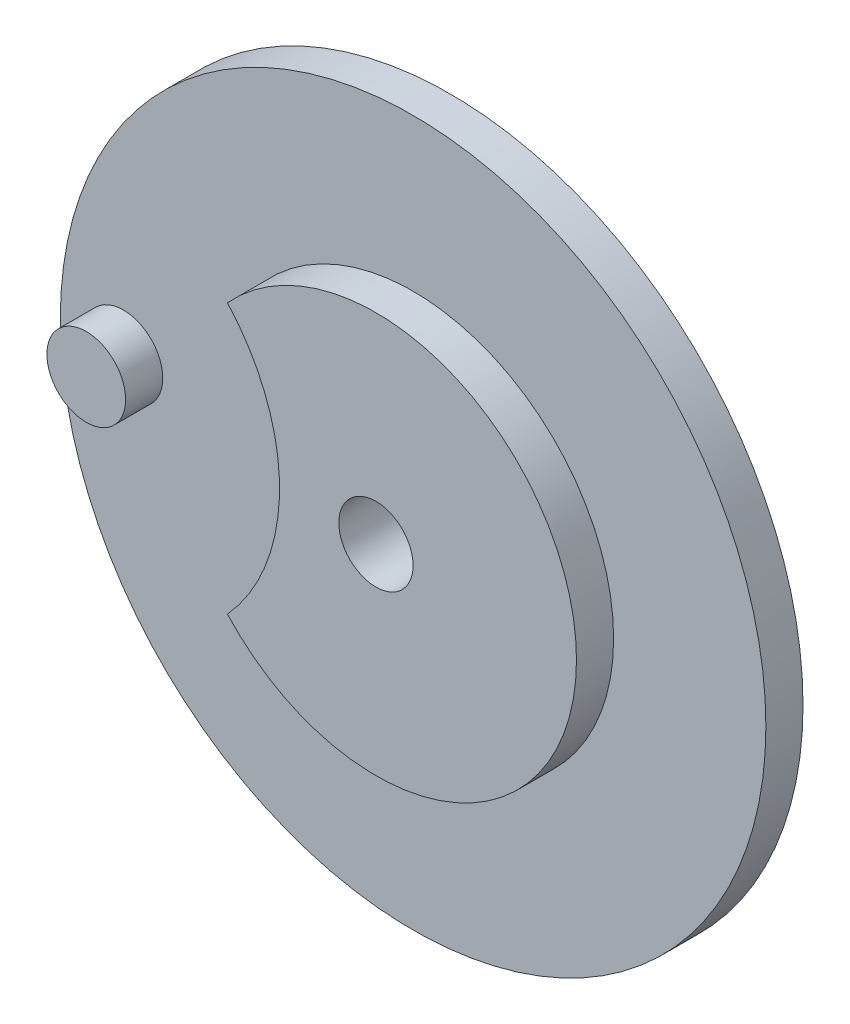
from build123d import *

# Parameters (mm, degrees)
DRIVE_WHEEL_PROFILE_R           = 47.5
DRIVE_WHEEL_PROFILE_R_2         = 5
DRIVE_DISC_95_DEPTH             = 5
LOCKING_START                   = 5
SKETCH1_3_R                     = 5
SKETCH1_3_R_2                   = 5.3
LOCKING_HUB_AND_DRIVE_PIN_DEPTH = 5


with BuildPart() as part:
    # Drive Wheel Profile → Drive Disc _95 (new body)
    with BuildSketch(Plane.XY):
        Circle(DRIVE_WHEEL_PROFILE_R)
        Circle(DRIVE_WHEEL_PROFILE_R_2, mode=Mode.SUBTRACT)
    extrude(amount=-DRIVE_DISC_95_DEPTH)

    # Sketch1_3 → Locking Hub and Drive Pin (add)
    # profile 1 of 2: a face of its own
    with BuildSketch(Plane.XY.offset(LOCKING_START)):
        with BuildLine():
            ThreePointArc((-19.989232296, -18.150222925), (-12.978464592, 0), (-19.989232296, 18.150222925))
            ThreePointArc((-19.989232296, 18.150222925), (27, 0), (-19.989232296, -18.150222925))
        make_face()
        Circle(SKETCH1_3_R, mode=Mode.SUBTRACT)
    # profile 2 of 2: a face of its own
    with BuildSketch(Plane.XY.offset(LOCKING_START)):
        with Locations((-39, 0)):
            Circle(SKETCH1_3_R_2)
    extrude(amount=-LOCKING_HUB_AND_DRIVE_PIN_DEPTH)


solid = part.part
